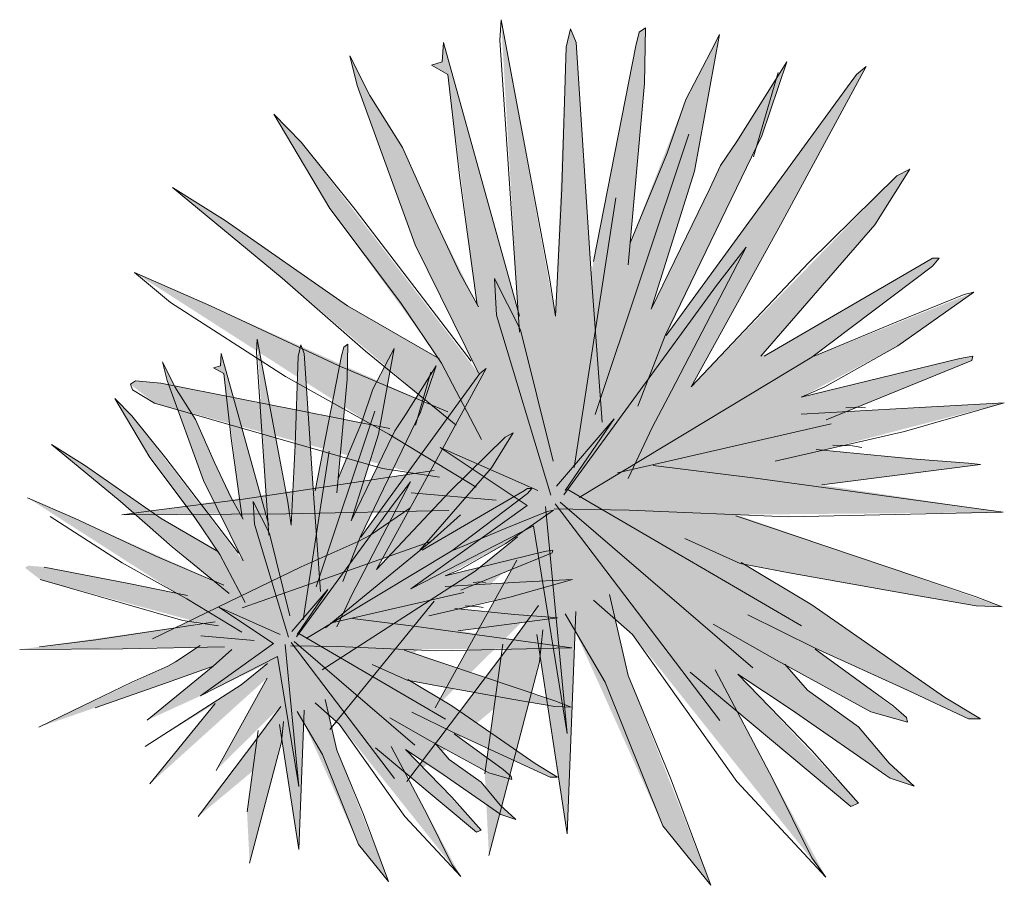
# Model space of a CAD drawing. Units: millimetres. Extents: x 595116 to 630915, y 909473 to 920225.
# Tile 1 of 134: x 595116 to 599072, y 909473 to 912950. Entities that reach past the tile are written whole.
import ezdxf

# ---------------------------------------------------------------- set-up
doc = ezdxf.new("R2010")
doc.units = ezdxf.units.MM
doc.layers.add('L-PLNT', color=85, linetype='Continuous', lineweight=13)

# ---------------------------------------------------------------- blocks, each defined once
blk = doc.blocks.new('A$C545C060E')
h = blk.add_hatch(color=256)
h.set_gradient(color1=(31, 127, 0), color2=(45, 179, 0), one_color=1, tint=0.35, name='INVSPHERICAL')
h.paths.add_polyline_path([(0.5289, 2.3933), (0.6449, 2.3037), (1.8889, 1.9675), (0.4886, 1.7698), (1.8427, 1.7866), (1.6176, 1.643), (0.6348, 1.1777), (1.0634, 1.3258), (1.9655, 1.643), (1.4613, 1.2308), (1.8689, 1.4167), (2.379, 1.6641), (2.1773, 1.5001), (1.4462, 1.0296), (1.9806, 1.3575), (1.4815, 0.7444), (2.376, 1.5525), (1.9861, 0.8479), (2.4798, 1.3362), (1.8495, 0.4957), (2.2655, 0.8421), (2.2227, 0.5329), (2.2428, 0.1416), (2.4875, 1.0934), (2.615, 0.2572), (2.6548, 1.2144), (3.074, 0.2836), (3.3026, 0), (2.9076, 1.0028), (2.8465, 1.2706), (2.9286, 1.1987), (3.8534, 0.0382), (3.4279, 0.8316), (3.9728, 0.3761), (4.0093, 0.3926), (3.4324, 1.0079), (3.9234, 0.6757), (4.1754, 0.507), (4.274, 0.4741), (4.1547, 0.583), (4.0093, 0.7573), (3.7652, 0.932), (3.6615, 1.0507), (4.0669, 0.8285), (4.2434, 0.7793), (4.2383, 0.801), (3.8017, 1.1334), (4.5341, 0.7955), (4.5913, 0.7955), (4.4198, 0.8993), (4.103, 1.1198), (3.7862, 1.3404), (3.4641, 1.5328), (3.9679, 1.4413), (4.4148, 1.3622), (4.5707, 1.3349), (4.6955, 1.3297), (3.9965, 1.5721), (3.4233, 1.7708), (4.6955, 1.7818), (3.8328, 1.9124), (4.5913, 2.0107), (3.836, 2.0787), (4.7056, 2.305), (3.9514, 2.2629), (4.5501, 2.5064), (4.5551, 2.5281), (4.493, 2.5174), (3.7341, 2.3322), (4.1967, 2.5773), (4.5602, 2.8334), (3.7862, 2.5226), (4.3627, 2.9585), (4.3942, 2.9967), (4.3627, 2.9967), (3.5576, 2.5281), (3.5488, 2.5358), (4.0875, 3.1548), (4.2539, 3.4216), (4.1913, 3.3889), (3.2093, 2.381), (4.0459, 3.9121), (3.9992, 3.874), (3.0899, 2.6261), (3.5471, 3.5797), (3.6664, 3.9338), (3.3496, 3.4381), (3.0173, 2.7516), (3.2248, 3.4109), (3.3446, 4.0644), (3.2433, 3.8685), (3.1836, 3.754), (2.9185, 3.073), (2.9862, 3.8303), (2.9912, 4.0971), (2.9601, 4.0754), (2.742, 2.9805), (2.7315, 2.9204), (2.6588, 4.0263), (2.6328, 4.0919), (2.6118, 4.0046), (2.5601, 2.7189), (2.3004, 4.1353), (2.3819, 2.7432), (2.0248, 4.0263), (2.0197, 3.9338), (1.9676, 3.9173), (2.0458, 3.874), (2.1853, 2.7764), (1.9756, 3.1968), (1.8294, 3.5244), (1.6731, 3.7731), (1.5773, 3.9632), (1.6126, 3.8206), (1.7512, 3.44), (1.8899, 3.0594), (2.1924, 2.4463), (1.3453, 3.5509), (1.2146, 3.6832), (1.4815, 3.2337), (2.0059, 2.5149), (1.5672, 2.7687), (0.9827, 3.1758), (0.7306, 3.3343), (1.255, 2.901), (1.9688, 2.2941), (0.9121, 2.7687), (0.5491, 2.9272), (1.6866, 2.1986), (0.6751, 2.3988), (0.5541, 2.4094)])
h = blk.add_hatch(color=256)
h.set_gradient(color1=(31, 127, 0), color2=(55, 219, 0), one_color=1, tint=0.43, name='SPHERICAL')
h.paths.add_polyline_path([(3.0231, 2.1876), (3.1143, 2.3616), (3.4711, 3.0487), (3.3303, 2.866), (2.6184, 1.8908), (2.6791, 1.8554), (2.9399, 2.0126)])
h = blk.add_hatch(color=256)
h.set_gradient(color1=(31, 127, 0), color2=(45, 179, 0), one_color=1, tint=0.35, name='INVSPHERICAL')
h.paths.add_polyline_path([(0.0253, 1.517), (0.0979, 1.4609), (0.8773, 1.2503), (0, 1.1265), (0.8483, 1.137), (0.7073, 1.047), (0.0916, 0.7555), (0.3601, 0.8483), (0.9253, 1.047), (0.6094, 0.7888), (0.8647, 0.9052), (1.1843, 1.0602), (1.0579, 0.9575), (0.5999, 0.6627), (0.9348, 0.8682), (0.622, 0.4841), (1.1825, 0.9903), (0.9382, 0.5489), (1.2475, 0.8548), (0.8526, 0.3283), (1.1132, 0.5452), (1.0864, 0.3516), (1.099, 0.1065), (1.2523, 0.7027), (1.3322, 0.1788), (1.3571, 0.7785), (1.6197, 0.1954), (1.7629, 0.0177), (1.5154, 0.6459), (1.4772, 0.8137), (1.5286, 0.7687), (2.108, 0.0416), (1.8414, 0.5387), (2.1827, 0.2533), (2.2057, 0.2637), (1.8442, 0.6492), (2.1518, 0.441), (2.3097, 0.3353), (2.3715, 0.3147), (2.2967, 0.383), (2.2057, 0.4922), (2.0527, 0.6016), (1.9878, 0.676), (2.2417, 0.5367), (2.3523, 0.5059), (2.3491, 0.5195), (2.0756, 0.7278), (2.5344, 0.5161), (2.5702, 0.5161), (2.4628, 0.5811), (2.2644, 0.7193), (2.0659, 0.8574), (1.8641, 0.978), (2.1797, 0.9206), (2.4597, 0.8711), (2.5573, 0.854), (2.6355, 0.8507), (2.1976, 1.0026), (1.8385, 1.1271), (2.6355, 1.134), (2.0951, 1.2158), (2.5702, 1.2774), (2.0971, 1.32), (2.6418, 1.4617), (2.1694, 1.4353), (2.5444, 1.5879), (2.5476, 1.6015), (2.5086, 1.5948), (2.0332, 1.4787), (2.3231, 1.6323), (2.5508, 1.7927), (2.0659, 1.5981), (2.427, 1.8711), (2.4468, 1.8951), (2.427, 1.8951), (1.9227, 1.6015), (1.9171, 1.6063), (2.2546, 1.9941), (2.3589, 2.1612), (2.3196, 2.1408), (1.7045, 1.5093), (2.2286, 2.4686), (2.1993, 2.4447), (1.6297, 1.6629), (1.9161, 2.2603), (1.9909, 2.4821), (1.7924, 2.1716), (1.5842, 1.7415), (1.7142, 2.1546), (1.7892, 2.564), (1.7258, 2.4412), (1.6884, 2.3695), (1.5223, 1.9429), (1.5647, 2.4173), (1.5678, 2.5844), (1.5484, 2.5709), (1.4117, 1.8849), (1.4052, 1.8472), (1.3596, 2.5401), (1.3433, 2.5812), (1.3301, 2.5265), (1.2978, 1.721), (1.1351, 2.6083), (1.1861, 1.7362), (0.9624, 2.5401), (0.9592, 2.4821), (0.9266, 2.4718), (0.9756, 2.4447), (1.0629, 1.7571), (0.9316, 2.0204), (0.84, 2.2257), (0.7421, 2.3814), (0.682, 2.5006), (0.7042, 2.4112), (0.791, 2.1728), (0.8779, 1.9344), (1.0674, 1.5503), (0.5367, 2.2423), (0.4549, 2.3251), (0.622, 2.0435), (0.9505, 1.5932), (0.6757, 1.7522), (0.3096, 2.0073), (0.1516, 2.1065), (0.4801, 1.8351), (0.9274, 1.4549), (0.2653, 1.7522), (0.0379, 1.8515), (0.7505, 1.3951), (0.1169, 1.5205), (0.0411, 1.5272)])
h = blk.add_hatch(color=256)
h.set_gradient(color1=(31, 127, 0), color2=(55, 219, 0), one_color=1, tint=0.43, name='SPHERICAL')
h.paths.add_polyline_path([(1.3343, 1.2022), (1.3723, 1.1801), (1.5357, 1.2786), (1.5878, 1.3882), (1.645, 1.4972), (1.8684, 1.9277), (1.7803, 1.8132)])
for p, q in [((2.2949, 4.0373, -52.7691), (2.3004, 4.1353, -52.7691)), ((2.3004, 4.1353, -52.7691), (2.534, 2.8932, -52.7691)), ((2.9601, 4.0754, -52.7691), (2.9912, 4.0971, -52.7691)), ((2.9912, 4.0971, -52.7691), (2.9862, 3.8303, -52.7691)), ((2.6118, 4.0046, -52.7691), (2.6328, 4.0919, -52.7691)), ((2.6328, 4.0919, -52.7691), (2.6588, 4.0263, -52.7691)), ((2.9446, 4.0101, -52.7691), (2.9601, 4.0754, -52.7691)), ((3.3446, 4.0644, -52.7691), (3.2248, 3.4109, -52.7691)), ((3.303, 3.983, -52.7691), (3.3446, 4.0644, -52.7691)), ((2.0197, 3.9338, -52.7691), (2.0248, 4.0263, -52.7691)), ((2.0248, 4.0263, -52.7691), (2.3887, 2.7189, -52.7691)), ((2.3887, 2.6426, -52.7691), (2.2949, 4.0373, -52.7691)), ((2.5912, 3.3291, -52.7691), (2.6118, 4.0046, -52.7691)), ((2.6588, 4.0263, -52.7691), (2.7315, 2.9204, -52.7691)), ((2.742, 2.9805, -52.7691), (2.9446, 4.0101, -52.7691)), ((1.5773, 3.9632, -52.7691), (1.6126, 3.8206, -52.7691)), ((1.6731, 3.7731, -52.7691), (1.5773, 3.9632, -52.7691)), ((3.1836, 3.754, -52.7691), (3.303, 3.983, -52.7691)), ((1.9676, 3.9173, -52.7691), (2.0197, 3.9338, -52.7691)), ((2.0458, 3.874, -52.7691), (1.9676, 3.9173, -52.7691)), ((3.4278, 3.5526, -52.7691), (3.6664, 3.9338, -52.7691)), ((3.6664, 3.9338, -52.7691), (3.5471, 3.5797, -52.7691)), ((4.0459, 3.9121, -52.7691), (3.6354, 3.1548, -52.7691)), ((3.9992, 3.874, -52.7691), (4.0459, 3.9121, -52.7691)), ((2.1029, 3.3779, -52.7691), (2.0458, 3.874, -52.7691)), ((3.5076, 3.4794, -52.7691), (3.6246, 3.8836, -52.7691)), ((3.5576, 3.269, -52.7691), (3.9992, 3.874, -52.7691)), ((1.6126, 3.8206, -52.7691), (1.8899, 3.0594, -52.7691)), ((2.9862, 3.8303, -52.7691), (2.908, 2.964, -52.7691)), ((1.8294, 3.5244, -52.7691), (1.6731, 3.7731, -52.7691)), ((3.095, 3.4979, -52.7691), (3.1836, 3.754, -52.7691)), ((1.2146, 3.6832, -52.7691), (1.4815, 3.2337, -52.7691)), ((1.3453, 3.5509, -52.7691), (1.2146, 3.6832, -52.7691)), ((3.1975, 3.5881, -52.7691), (2.7496, 2.2484, -52.7691)), ((3.5471, 3.5797, -52.7691), (3.0849, 2.6261, -52.7691)), ((1.6025, 3.2285, -52.7691), (1.3453, 3.5509, -52.7691)), ((3.3496, 3.4381, -52.7691), (3.4278, 3.5526, -52.7691)), ((1.9756, 3.1968, -52.7691), (1.8294, 3.5244, -52.7691)), ((2.9185, 3.073, -52.7691), (3.095, 3.4979, -52.7691)), ((3.2979, 3.3291, -52.7691), (3.3496, 3.4381, -52.7691)), ((3.2248, 3.4109, -52.7691), (3.0173, 2.7516, -52.7691)), ((3.7707, 2.975, -52.7691), (4.1913, 3.3889, -52.7691)), ((4.2539, 3.4216, -52.7691), (4.0875, 3.1548, -52.7691)), ((4.1913, 3.3889, -52.7691), (4.2539, 3.4216, -52.7691)), ((2.1857, 2.7732, -52.7691), (2.1029, 3.3779, -52.7691)), ((0.7306, 3.3343, -52.7691), (1.255, 2.901, -52.7691)), ((0.9827, 3.1758, -52.7691), (0.7306, 3.3343, -52.7691)), ((2.5601, 2.7189, -52.7691), (2.5912, 3.3291, -52.7691)), ((3.0173, 2.7516, -52.7691), (3.2979, 3.3291, -52.7691)), ((2.8492, 3.2835, -52.7691), (2.65, 1.9962, -52.7691)), ((3.0899, 2.6261, -52.7691), (3.5576, 3.269, -52.7691)), ((1.4815, 3.2337, -52.7691), (1.8193, 2.7845, -52.7691)), ((2.1571, 2.5045, -52.7691), (1.6025, 3.2285, -52.7691)), ((1.5672, 2.7687, -52.7691), (0.9827, 3.1758, -52.7691)), ((2.1017, 2.9272, -52.7691), (1.9756, 3.1968, -52.7691)), ((3.6354, 3.1548, -52.7691), (3.2093, 2.381, -52.7691)), ((4.0875, 3.1548, -52.7691), (3.5421, 2.5281, -52.7691)), ((1.8899, 3.0594, -52.7691), (2.1924, 2.4463, -52.7691)), ((3.4711, 3.0487, -52.7691), (3.1143, 2.3616, -52.7691)), ((3.3303, 2.866, -52.7691), (3.4711, 3.0487, -52.7691)), ((3.2093, 2.381, -52.7691), (3.7707, 2.975, -52.7691)), ((3.5576, 2.5281, -52.7691), (4.3266, 2.975, -52.7691)), ((4.3266, 2.975, -52.7691), (4.3627, 2.9967, -52.7691)), ((4.3942, 2.9967, -52.7691), (4.3627, 2.9585, -52.7691)), ((4.3627, 2.9967, -52.7691), (4.3942, 2.9967, -52.7691)), ((0.5491, 2.9272, -52.7691), (0.7205, 2.7845, -52.7691)), ((0.9121, 2.7687, -52.7691), (0.5491, 2.9272, -52.7691)), ((2.1924, 2.7635, -52.7691), (2.1017, 2.9272, -52.7691)), ((2.7315, 2.9204, -52.7691), (2.7832, 2.2122, -52.7691)), ((4.3627, 2.9585, -52.7691), (3.7862, 2.5226, -52.7691)), ((1.255, 2.901, -52.7691), (1.6529, 2.552, -52.7691)), ((2.2689, 2.8987, -52.7691), (2.3937, 2.6536, -52.7691)), ((2.2794, 2.7244, -52.7691), (2.2689, 2.8987, -52.7691)), ((2.534, 2.8932, -52.7691), (2.5601, 2.7189, -52.7691)), ((2.6, 1.8655, -52.7691), (3.3303, 2.866, -52.7691)), ((4.5602, 2.8334, -52.7691), (4.1967, 2.5773, -52.7691)), ((4.5135, 2.8224, -52.7691), (4.5602, 2.8334, -52.7691)), ((0.7205, 2.7845, -52.7691), (1.2701, 2.4305, -52.7691)), ((1.8193, 2.7845, -52.7691), (2.0159, 2.4938, -52.7691)), ((4.1913, 2.6917, -52.7691), (4.5135, 2.8224, -52.7691)), ((1.5218, 2.4832, -52.7691), (0.9121, 2.7687, -52.7691)), ((2.0059, 2.5149, -52.7691), (1.5672, 2.7687, -52.7691)), ((2.5391, 1.8636, -52.7691), (2.2794, 2.7244, -52.7691)), ((3.7967, 2.5281, -52.7691), (4.1913, 2.6917, -52.7691)), ((2.3937, 2.6536, -52.7691), (2.5496, 2.0269, -52.7691)), ((1.1317, 2.547), (1.1351, 2.6083)), ((1.1351, 2.6083), (1.2814, 1.8302)), ((3.0849, 2.6261, -52.7691), (2.9546, 2.2885, -52.7691)), ((1.1904, 1.6732), (1.1317, 2.547)), ((1.3301, 2.5265), (1.3433, 2.5812)), ((1.3433, 2.5812), (1.3596, 2.5401)), ((1.5386, 2.5299), (1.5484, 2.5709)), ((1.5484, 2.5709), (1.5678, 2.5844)), ((1.5678, 2.5844), (1.5647, 2.4173)), ((1.6529, 2.552, -52.7691), (2.0865, 2.198, -52.7691)), ((1.7892, 2.564), (1.7142, 2.1546)), ((1.7632, 2.5129), (1.7892, 2.564)), ((4.1967, 2.5773, -52.7691), (3.8484, 2.381, -52.7691)), ((0.682, 2.5006), (0.7042, 2.4112)), ((0.7421, 2.3814), (0.682, 2.5006)), ((0.9592, 2.4821), (0.9624, 2.5401)), ((0.9624, 2.5401), (1.1904, 1.721)), ((1.3172, 2.1033), (1.3301, 2.5265)), ((1.3596, 2.5401), (1.4052, 1.8472)), ((1.4117, 1.8849), (1.5386, 2.5299)), ((1.6884, 2.3695), (1.7632, 2.5129)), ((3.7862, 2.5226, -52.7691), (2.6744, 1.8526, -52.7691)), ((3.7341, 2.3322, -52.7691), (4.493, 2.5174, -52.7691)), ((4.5501, 2.5064, -52.7691), (3.8539, 2.2232, -52.7691)), ((4.493, 2.5174, -52.7691), (4.5551, 2.5281, -52.7691)), ((4.5551, 2.5281, -52.7691), (4.5501, 2.5064, -52.7691)), ((0.9266, 2.4718), (0.9592, 2.4821)), ((0.9756, 2.4447), (0.9266, 2.4718)), ((2.0462, 2.2613, -52.7691), (1.5218, 2.4832, -52.7691)), ((1.8413, 2.2433), (1.9909, 2.4821)), ((1.8914, 2.1975), (1.9646, 2.4507)), ((1.9909, 2.4821), (1.9161, 2.2603)), ((2.2286, 2.4686), (1.9714, 1.9941)), ((2.0159, 2.4938, -52.7691), (2.2075, 2.1291, -52.7691)), ((2.1993, 2.4447), (2.2286, 2.4686)), ((0.5541, 2.4094, -52.7691), (0.5289, 2.3933, -52.7691)), ((0.6751, 2.3988, -52.7691), (0.5541, 2.4094, -52.7691)), ((0.7042, 2.4112), (0.8779, 1.9344)), ((1.0114, 2.1339), (0.9756, 2.4447)), ((1.2701, 2.4305, -52.7691), (1.7638, 2.1556, -52.7691)), ((1.5647, 2.4173), (1.5157, 1.8746)), ((1.9227, 2.0656), (2.1993, 2.4447)), ((0.5289, 2.3933, -52.7691), (0.539, 2.3671, -52.7691)), ((0.539, 2.3671, -52.7691), (0.6449, 2.3037, -52.7691)), ((1.3201, 2.272, -52.7691), (0.6751, 2.3988, -52.7691)), ((0.84, 2.2257), (0.7421, 2.3814)), ((1.6329, 2.2091), (1.6884, 2.3695)), ((3.1143, 2.3616, -52.7691), (3.0231, 2.1876, -52.7691)), ((3.8484, 2.381, -52.7691), (3.7341, 2.3322, -52.7691)), ((0.4549, 2.3251), (0.622, 2.0435)), ((0.5367, 2.2423), (0.4549, 2.3251)), ((0.6449, 2.3037, -52.7691), (1.7336, 1.9916, -52.7691)), ((1.7689, 2.1821, -52.7691), (1.3201, 2.272, -52.7691)), ((1.6971, 2.2656), (1.4165, 1.4263)), ((1.9161, 2.2603), (1.6265, 1.6629)), ((3.7341, 2.2503, -52.7691), (4.3005, 2.283, -52.7691)), ((3.9485, 2.2815, -52.7691), (4.0007, 2.2849, -52.7691)), ((4.0007, 2.2849, -52.7691), (4.0421, 2.2815, -52.7691)), ((4.7056, 2.305, -52.7691), (4.2278, 2.1685, -52.7691)), ((4.3005, 2.283, -52.7691), (4.7056, 2.305, -52.7691)), ((0.6978, 2.0403), (0.5367, 2.2423)), ((0.9316, 2.0204), (0.84, 2.2257)), ((1.7924, 2.1716), (1.8413, 2.2433)), ((2.5647, 1.9069, -52.7691), (2.8404, 2.2287, -52.7691)), ((2.8404, 2.2287, -52.7691), (2.6063, 1.8853, -52.7691)), ((1.5223, 1.9429), (1.6329, 2.2091)), ((1.76, 2.1033), (1.7924, 2.1716)), ((3.8778, 2.2051, -52.7691), (2.8572, 1.97, -52.7691)), ((3.0231, 2.1876, -52.7691), (2.9072, 1.9438, -52.7691)), ((4.2278, 2.1685, -52.7691), (3.6097, 2.0269, -52.7691)), ((1.0632, 1.7551), (1.0114, 2.1339)), ((1.7142, 2.1546), (1.5842, 1.7415)), ((1.7638, 2.1556, -52.7691), (2.1823, 1.9017, -52.7691)), ((2.0561, 1.8815), (2.3196, 2.1408)), ((2.3589, 2.1612), (2.2546, 1.9941)), ((2.3196, 2.1408), (2.3589, 2.1612)), ((0.1516, 2.1065), (0.4801, 1.8351)), ((0.3096, 2.0073), (0.1516, 2.1065)), ((1.2978, 1.721), (1.3172, 2.1033)), ((1.4789, 2.0747), (1.3541, 1.2683)), ((1.5842, 1.7415), (1.76, 2.1033)), ((2.0088, 2.0922, -52.7691), (2.4765, 1.8853, -52.7691)), ((2.4248, 1.8144, -52.7691), (2.0088, 2.0922, -52.7691)), ((3.8068, 2.0815, -52.7691), (4.264, 2.0379, -52.7691)), ((3.8857, 2.1023, -52.7691), (3.9797, 2.0989, -52.7691)), ((3.9797, 2.0989, -52.7691), (4.025, 2.0914, -52.7691)), ((0.622, 2.0435), (0.8337, 1.7622)), ((1.0453, 1.5867), (0.6978, 2.0403)), ((1.6297, 1.6629), (1.9227, 2.0656)), ((4.264, 2.0379, -52.7691), (4.5341, 2.0162, -52.7691)), ((0.6757, 1.7522), (0.3096, 2.0073)), ((1.0106, 1.8515), (0.9316, 2.0204)), ((1.9806, 1.9813, -52.7691), (1.0684, 1.8439, -52.7691)), ((1.9714, 1.9941), (1.7045, 1.5093)), ((1.7336, 1.9916, -52.7691), (2.0059, 1.9493, -52.7691)), ((2.2546, 1.9941), (1.9129, 1.6015)), ((3.516, 1.9454, -52.7691), (3.0278, 2.0052, -52.7691)), ((4.5913, 2.0107, -52.7691), (3.8328, 1.9124, -52.7691)), ((4.5341, 2.0162, -52.7691), (4.5913, 2.0107, -52.7691)), ((0.8779, 1.9344), (1.0674, 1.5503)), ((4.7005, 1.7818, -52.7691), (3.516, 1.9454, -52.7691)), ((1.8684, 1.9277), (1.645, 1.4972)), ((1.7803, 1.8132), (1.8684, 1.9277)), ((2.4044, 1.8815), (2.427, 1.8951)), ((2.4468, 1.8951), (2.427, 1.8711)), ((2.427, 1.8951), (2.4468, 1.8951)), ((3.7366, 1.2392, -52.7691), (2.6168, 1.8917, -52.7691)), ((0.2653, 1.7522), (0.0379, 1.8515)), ((1.0684, 1.8439, -52.7691), (0.6398, 1.7908, -52.7691)), ((1.0674, 1.749), (1.0106, 1.8515)), ((1.4052, 1.8472), (1.4375, 1.4036)), ((1.7045, 1.5093), (2.0561, 1.8815)), ((1.8701, 1.8743, -52.7691), (2.2765, 1.8397, -52.7691)), ((1.9227, 1.6015), (2.4044, 1.8815)), ((2.427, 1.8711), (2.0659, 1.5981)), ((0.4801, 1.8351), (0.7294, 1.6165)), ((0.6398, 1.7908, -52.7691), (0.4886, 1.7698, -52.7691)), ((1.1153, 1.8337), (1.1935, 1.6801)), ((1.1219, 1.7245), (1.1153, 1.8337)), ((1.2751, 1.775, -52.7691), (2.0512, 1.7908, -52.7691)), ((1.2814, 1.8302), (1.2978, 1.721)), ((1.3228, 1.1864), (1.7803, 1.8132)), ((1.8647, 1.8015, -52.7691), (1.6781, 1.6747, -52.7691)), ((1.8689, 1.4167, -52.7691), (2.4248, 1.8144, -52.7691)), ((2.5508, 1.7927), (2.3231, 1.6323)), ((2.513, 1.8089, -52.7691), (2.6168, 0.7247, -52.7691)), ((2.5215, 1.7859), (2.5508, 1.7927)), ((2.9135, 1.7928, -52.7691), (2.5546, 1.7983, -52.7691)), ((3.3467, 0.7868, -52.7691), (2.5588, 1.8222, -52.7691)), ((3.5043, 1.0393, -52.7691), (2.5836, 1.8309, -52.7691)), ((3.6719, 1.7601, -52.7691), (2.9135, 1.7928, -52.7691)), ((0.1453, 1.7622), (0.4896, 1.5403)), ((0.6473, 1.5733), (0.2653, 1.7522)), ((0.4886, 1.7698, -52.7691), (1.2751, 1.775, -52.7691)), ((0.9505, 1.5932), (0.6757, 1.7522)), ((0.8337, 1.7622), (0.9569, 1.58)), ((1.9655, 1.643, -52.7691), (2.1067, 1.7698, -52.7691)), ((2.3196, 1.704), (2.5215, 1.7859)), ((3.4223, 1.7656, -52.7691), (4.5707, 1.3785, -52.7691)), ((4.6955, 1.7818, -52.7691), (3.6719, 1.7601, -52.7691)), ((1.2846, 1.1852), (1.1219, 1.7245)), ((2.4559, 1.7165, -52.7691), (1.8689, 1.4167, -52.7691)), ((2.0725, 1.6015), (2.3196, 1.704)), ((2.6168, 0.7247, -52.7691), (2.4559, 1.7165, -52.7691)), ((1.1935, 1.6801), (1.2912, 1.2875)), ((1.6265, 1.6629), (1.5449, 1.4514)), ((1.6781, 1.6747, -52.7691), (1.6176, 1.643, -52.7691)), ((2.1773, 1.5001, -52.7691), (2.379, 1.6641, -52.7691)), ((3.4433, 1.5367, -52.7691), (3.1782, 1.6566, -52.7691)), ((0.7294, 1.6165), (1.0011, 1.3947)), ((1.6176, 1.643, -52.7691), (1.3453, 1.5215, -52.7691)), ((1.9655, 1.643, -52.7691), (1.4613, 1.2308, -52.7691)), ((1.6075, 1.516, -52.7691), (1.9655, 1.643, -52.7691)), ((2.3231, 1.6323), (2.1048, 1.5093)), ((2.5086, 1.5948), (2.5476, 1.6015)), ((2.5476, 1.6015), (2.5444, 1.5879)), ((0.9758, 1.4344), (0.6473, 1.5733)), ((0.9569, 1.58), (1.0769, 1.3515)), ((2.0659, 1.5981), (1.3694, 1.1783)), ((2.0332, 1.4787), (2.5086, 1.5948)), ((2.5444, 1.5879), (2.1083, 1.4105)), ((0.5209, 1.4411), (0.1169, 1.5205)), ((0.4896, 1.5403), (0.7989, 1.3681)), ((1.3453, 1.5215, -52.7691), (1.0482, 1.3785, -52.7691)), ((1.0634, 1.3258, -52.7691), (1.6075, 1.516, -52.7691)), ((1.9861, 0.8479, -52.7691), (2.376, 1.5525, -52.7691)), ((2.1048, 1.5093), (2.0332, 1.4787)), ((3.677, 1.493, -52.7691), (3.4433, 1.5367, -52.7691)), ((3.4484, 1.5422, -52.7691), (3.7862, 1.3404, -52.7691)), ((0.0979, 1.4609), (0.78, 1.2654)), ((1.4462, 1.0296, -52.7691), (2.1773, 1.5001, -52.7691)), ((1.645, 1.4972), (1.5878, 1.3882)), ((2.6418, 1.4617), (2.3425, 1.3762)), ((2.3881, 1.448), (2.6418, 1.4617)), ((4.2589, 1.3895, -52.7691), (3.677, 1.493, -52.7691)), ((0.8021, 1.3847), (0.5209, 1.4411)), ((1.3006, 1.2124), (1.4733, 1.4139)), ((1.4733, 1.4139), (1.3267, 1.1988)), ((2.0332, 1.4275), (2.3881, 1.448)), ((2.1676, 1.447), (2.2002, 1.4491)), ((2.2002, 1.4491), (2.2262, 1.447)), ((1.0482, 1.3785, -52.7691), (0.6348, 1.1777, -52.7691)), ((0.7989, 1.3681), (1.0611, 1.2091)), ((2.1233, 1.3991), (1.4839, 1.2519)), ((1.5878, 1.3882), (1.5152, 1.2354)), ((2.3425, 1.3762), (1.9553, 1.2875)), ((2.8193, 1.3895, -52.7691), (2.9076, 1.0028, -52.7691)), ((4.5707, 1.3349, -52.7691), (4.2589, 1.3895, -52.7691)), ((4.5707, 1.3785, -52.7691), (4.6955, 1.3297, -52.7691)), ((0.9524, 1.3284), (1.2454, 1.1988)), ((1.213, 1.1544), (0.9524, 1.3284)), ((1.9806, 1.3575, -52.7691), (1.4815, 0.7444, -52.7691)), ((2.0788, 1.3217), (2.3652, 1.2944)), ((2.1282, 1.3348), (2.1871, 1.3326)), ((2.1871, 1.3326), (2.2155, 1.3279)), ((2.3134, 1.1092, -52.7691), (2.4798, 1.3362, -52.7691)), ((2.9286, 1.1987, -52.7691), (2.7416, 1.3624, -52.7691)), ((3.7862, 1.3404, -52.7691), (4.4198, 0.8993, -52.7691)), ((4.6955, 1.3297, -52.7691), (4.5707, 1.3349, -52.7691)), ((1.8966, 1.2365), (1.5907, 1.2739)), ((2.5702, 1.2774), (2.0951, 1.2158)), ((2.3652, 1.2944), (2.5344, 1.2808)), ((2.5344, 1.2808), (2.5702, 1.2774)), ((2.7988, 0.9698, -52.7691), (2.6063, 1.2967, -52.7691)), ((2.6584, 1.3077, -52.7691), (2.6168, 0.2454, -52.7691)), ((3.8017, 1.1334, -52.7691), (3.4795, 1.2915, -52.7691)), ((0.9348, 1.2589), (0.3633, 1.1728)), ((0.78, 1.2654), (0.9505, 1.2389)), ((2.6387, 1.134), (1.8966, 1.2365)), ((3.6198, 1.0736, -52.7691), (3.3135, 1.2479, -52.7691)), ((0.8655, 1.1919), (1.1201, 1.1702)), ((2.0348, 0.794), (1.3333, 1.2028)), ((2.6168, 0.2454, -52.7691), (2.4714, 1.1987, -52.7691)), ((2.4849, 1.0668, -52.7691), (2.5, 1.2201, -52.7691)), ((3.4274, 0.496, -52.7691), (2.9286, 1.1987, -52.7691)), ((0, 1.1265), (0.4928, 1.1297)), ((0.3633, 1.1728), (0.0948, 1.1396)), ((0.4928, 1.1297), (0.979, 1.1396)), ((0.8621, 1.1463), (0.7452, 1.0669)), ((0.8647, 0.9052), (1.213, 1.1544)), ((1.2683, 1.151), (1.3333, 0.4717)), ((1.5191, 1.1408), (1.2943, 1.1443)), ((1.7905, 0.5106), (1.297, 1.1593)), ((1.8892, 0.6688), (1.3125, 1.1647)), ((1.9943, 1.1204), (1.5191, 1.1408)), ((2.6355, 1.134), (1.9943, 1.1204)), ((2.3084, 1.1512, -52.7691), (2.2227, 0.5329, -52.7691)), ((4.2434, 0.932, -52.7691), (3.8017, 1.1334, -52.7691)), ((1.2325, 1.093), (0.8647, 0.9052)), ((0.9253, 1.047), (1.0137, 1.1265)), ((1.3333, 0.4717), (1.2325, 1.093)), ((1.8379, 1.1238), (2.5573, 0.8813)), ((1.8495, 0.4957, -52.7691), (2.3134, 1.1092, -52.7691)), ((3.8017, 1.1279, -52.7691), (4.1757, 0.8556, -52.7691)), ((0.7073, 1.047), (0.5367, 0.9709)), ((0.9253, 1.047), (0.6094, 0.7888)), ((0.701, 0.9674), (0.9253, 1.047)), ((0.7452, 1.0669), (0.7073, 1.047)), ((1.0579, 0.9575), (1.1843, 1.0602)), ((1.8511, 0.9804), (1.685, 1.0556)), ((2.2428, 0.1416, -52.7691), (2.4849, 1.0668, -52.7691)), ((4.0669, 0.8285, -52.7691), (3.6198, 1.0736, -52.7691)), ((3.6559, 1.0571, -52.7691), (3.7652, 0.932, -52.7691)), ((0.9382, 0.5489), (1.1825, 0.9903)), ((2.9076, 1.0028, -52.7691), (3.1105, 0.5122, -52.7691)), ((3.9728, 0.3761, -52.7691), (3.2038, 1.0189, -52.7691)), ((3.3236, 1.0299, -52.7691), (3.5988, 0.5067, -52.7691)), ((3.687, 0.8391, -52.7691), (3.4324, 1.0079, -52.7691)), ((3.4324, 1.0079, -52.7691), (3.7858, 0.6432, -52.7691)), ((0.5367, 0.9709), (0.3506, 0.8813)), ((0.3601, 0.8483), (0.701, 0.9674)), ((0.5999, 0.6627), (1.0579, 0.9575)), ((1.9974, 0.953), (1.8511, 0.9804)), ((1.8542, 0.9838), (2.0659, 0.8574)), ((2.362, 0.8882), (1.9974, 0.953)), ((3.074, 0.2836, -52.7691), (2.7988, 0.9698, -52.7691)), ((3.7652, 0.932, -52.7691), (4.0093, 0.7573, -52.7691)), ((4.5341, 0.7955, -52.7691), (4.2434, 0.932, -52.7691)), ((4.4198, 0.8993, -52.7691), (4.5913, 0.7955, -52.7691)), ((0.3506, 0.8813), (0.0916, 0.7555)), ((0.9348, 0.8682), (0.622, 0.4841)), ((1.1432, 0.7126), (1.2475, 0.8548)), ((1.5286, 0.7687), (1.4115, 0.8712)), ((1.4602, 0.8882), (1.5154, 0.6459)), ((2.0659, 0.8574), (2.4628, 0.5811)), ((2.5573, 0.854), (2.362, 0.8882)), ((2.5573, 0.8813), (2.6355, 0.8507)), ((2.6355, 0.8507), (2.5573, 0.854)), ((4.1757, 0.8556, -52.7691), (4.2383, 0.801, -52.7691)), ((1.4473, 0.6253), (1.3267, 0.8301)), ((1.3594, 0.837), (1.3333, 0.1715)), ((2.0756, 0.7278), (1.8737, 0.8268)), ((4.1597, 0.5122, -52.7691), (3.687, 0.8391, -52.7691)), ((4.2434, 0.7793, -52.7691), (4.0669, 0.8285, -52.7691)), ((4.2383, 0.801, -52.7691), (4.2434, 0.7793, -52.7691)), ((1.3333, 0.1715), (1.2422, 0.7687)), ((1.2506, 0.686), (1.2601, 0.7821)), ((1.8411, 0.3285), (1.5286, 0.7687)), ((1.9616, 0.6903), (1.7697, 0.7995)), ((4.0093, 0.7573, -52.7691), (4.1547, 0.583, -52.7691)), ((4.5913, 0.7955, -52.7691), (4.5341, 0.7955, -52.7691)), ((0.8526, 0.3283), (1.1432, 0.7126)), ((1.1401, 0.7389), (1.0864, 0.3516)), ((2.3523, 0.6016), (2.0756, 0.7278)), ((2.0756, 0.7243), (2.3099, 0.5538)), ((1.099, 0.1065), (1.2506, 0.686)), ((1.7761, 0.6629), (1.9485, 0.3352)), ((2.2417, 0.5367), (1.9616, 0.6903)), ((1.9843, 0.68), (2.0527, 0.6016)), ((1.6197, 0.1954), (1.4473, 0.6253)), ((1.5154, 0.6459), (1.6426, 0.3386)), ((2.1827, 0.2533), (1.701, 0.6561)), ((2.0037, 0.5434), (1.8442, 0.6492)), ((1.8442, 0.6492), (2.0656, 0.4207)), ((3.7858, 0.6432, -52.7691), (4.0093, 0.3926, -52.7691)), ((2.0527, 0.6016), (2.2057, 0.4922)), ((2.5344, 0.5161), (2.3523, 0.6016)), ((2.4628, 0.5811), (2.5702, 0.5161)), ((4.1547, 0.583, -52.7691), (4.274, 0.4741, -52.7691)), ((2.2999, 0.3386), (2.0037, 0.5434)), ((2.3523, 0.5059), (2.2417, 0.5367)), ((2.3099, 0.5538), (2.3491, 0.5195)), ((2.3491, 0.5195), (2.3523, 0.5059)), ((2.2057, 0.4922), (2.2967, 0.383)), ((2.5702, 0.5161), (2.5344, 0.5161)), ((3.1105, 0.5122, -52.7691), (3.3026, 0, -52.7691)), ((3.8534, 0.0382, -52.7691), (3.4274, 0.496, -52.7691)), ((3.5988, 0.5067, -52.7691), (3.7858, 0.131, -52.7691)), ((4.274, 0.4741, -52.7691), (4.1597, 0.5122, -52.7691)), ((2.0656, 0.4207), (2.2057, 0.2637)), ((2.2967, 0.383), (2.3715, 0.3147)), ((4.0093, 0.3926, -52.7691), (3.9728, 0.3761, -52.7691)), ((1.6426, 0.3386), (1.7629, 0.0177)), ((1.9485, 0.3352), (2.0656, 0.0998)), ((2.3715, 0.3147), (2.2999, 0.3386)), ((2.108, 0.0416), (1.8411, 0.3285)), ((3.3026, 0, -52.7691), (3.074, 0.2836, -52.7691)), ((2.2057, 0.2637), (2.1827, 0.2533)), ((1.7629, 0.0177), (1.6197, 0.1954)), ((2.0656, 0.0998), (2.108, 0.0416)), ((3.7858, 0.131, -52.7691), (3.8534, 0.0382, -52.7691))]:
    blk.add_line(p, q)

msp = doc.modelspace()

# ---------------------------------------------------------------- block references
at = {"layer": 'L-PLNT', "xscale": 840.7702618470988, "yscale": 840.7702618470988, "zscale": 840.7702618470988}
msp.add_blockref('A$C545C060E', (595115.631, 909473.208), dxfattribs=at)

doc.saveas('drawing.dxf')
